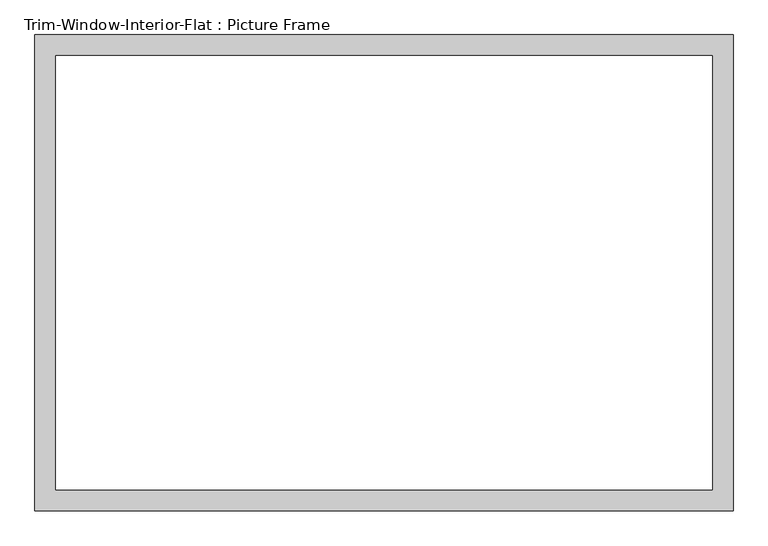
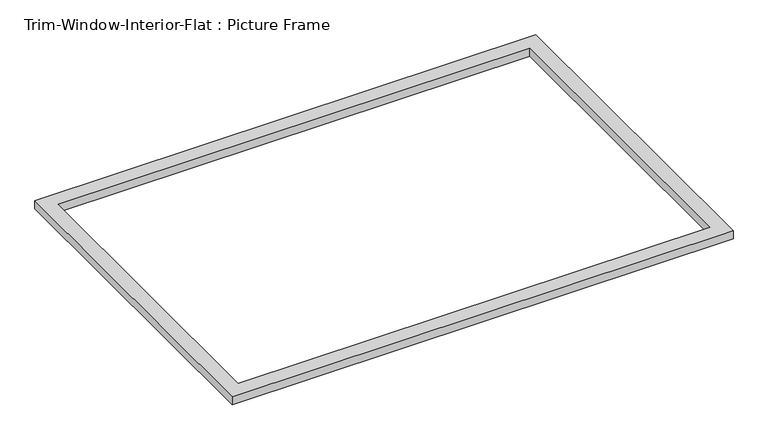
"""IFC4 building model written with IfcOpenShell, lengths in millimetres: proxy geometry, Trim-Window-Interior-Flat : Picture Frame."""

from ifc_helpers import new_model, si_unit, origin, origin_with_axes, place, context, project, spatial, polyline, outline, extrude, source, transform, mapped, element, save


def trim_window_interior_flat_picture_frame_03e64d7c(model_context):
    return source(origin(), model_context, "Body", "SweptSolid", [
        extrude(outline(polyline([(958.85, 44.45), (958.85, -1263.65), (-958.85, -1263.65), (-958.85, 44.45), (958.85, 44.45)]), holes=[polyline([(901.7, -12.7), (-901.7, -12.7), (-901.7, -1206.5), (901.7, -1206.5), (901.7, -12.7)])]), origin_with_axes(), (0.0, 0.0, 1.0), 31.75),
    ])


if __name__ == "__main__":
    model = new_model("IFC4")
    model_context = context("Model", 3, world=origin())
    ifc_project = project(units=[si_unit("LENGTHUNIT", "METRE", prefix="MILLI")], contexts=[model_context])
    site = spatial("IfcSite", under=ifc_project)
    building = spatial("IfcBuilding", under=site)
    placement = place(None, origin())
    trim_window_interior_flat_picture_frame_shape = trim_window_interior_flat_picture_frame_03e64d7c(model_context)
    element("IfcBuildingElementProxy", 1, Name="Trim-Window-Interior-Flat : Picture Frame", ObjectType="Trim-Window-Interior-Flat : Picture Frame", at=placement, inside=building, context=model_context, shape_type="MappedRepresentation", body=[
        mapped(trim_window_interior_flat_picture_frame_shape, transform((0.0, 0.0, 0.0), x_axis=(1.0, 0.0, 0.0), y_axis=(0.0, 1.0, 0.0), z_axis=(0.0, 0.0, 1.0))),
    ])
    save(model, "model.ifc")

# Revit data of these elements
# Type "Trim-Window-Interior-Flat : Picture Frame"
#   Trim Thickness_Picture Frame = 0' - 1 1/4"
#   Trim Width = 0' - 2 1/4"
#   Trim Thickness_with Sill = 0' - 0 3/4"
#   Sill Thickness = 0' - 1 1/4"
#   Opening Width [instance default] = 2' - 0"
#   Opening Height [instance default] = 3' - 0"
#   Default Elevation = 4' - 0"
#   Sill = no
#   Picture Frame = yes
#   Trim Material [instance default] = none
# Element 1 (IfcBuildingElementProxy, "Trim-Window-Interior-Flat : Picture Frame")
#   Opening Width = 6' - 0"
#   Opening Height = 4' - 0"
#   Trim Material = Wood - Stained
#   Materials on its faces: "Wood - Stained"
# Materials
#   "Wood - Stained": class "Wood", colour RGB 224 178 126, transparency 0, Cost = 0
